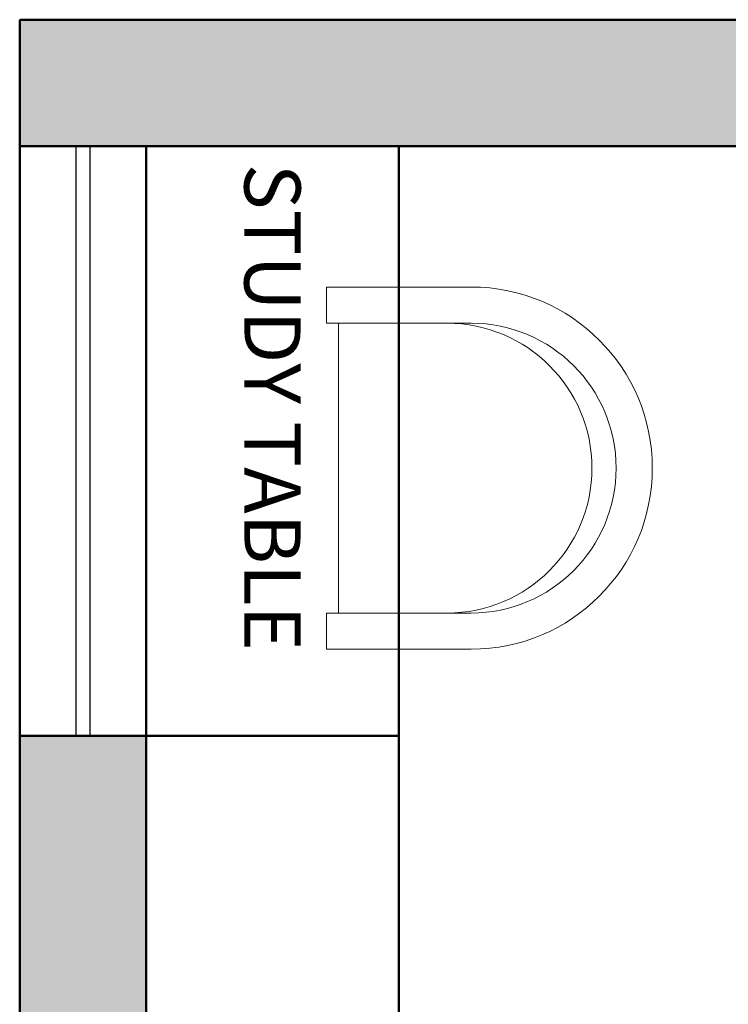
# Model space of a CAD drawing. Units: inches. Extents: x 3008 to 4088, y 1255 to 2137.
# Tile 17 of 30: x 3094 to 3144, y 1874 to 1944. Entities that reach past the tile are written whole.
import ezdxf

# ---------------------------------------------------------------- set-up
doc = ezdxf.new("R2010")
doc.units = ezdxf.units.IN
for name, color, linetype, lineweight in [('A-ANNO-TEXT', 7, 'Continuous', 18), ('A-FURN', 8, 'Continuous', 18), ('A-GLAZ', 4, 'Continuous', 25), ('A-WALL', 7, 'Continuous', 50), ('A-WALL-PATT', 8, 'Continuous', 13)]:
    doc.layers.add(name, color=color, linetype=linetype, lineweight=lineweight)
doc.styles.get("Standard").update_dxf_attribs({"font": 'arial.ttf'})

# ---------------------------------------------------------------- blocks, each defined once
blk = doc.blocks.new('12PSTG07')
at = {"color": 0, "linetype": 'ByBlock'}
for p, q in [((0, 15), (-12, 15)), ((0, 12), (0, 15)), ((-12, 12), (0, 12)), ((-1, -12), (-1, 12)), ((-12, -12), (0, -12)), ((0, -12), (0, -15)), ((0, -15), (-12, -15))]:
    blk.add_line(p, q, dxfattribs=at)
for centre, radius in [((-12, 0), 15), ((-12, 0), 12), ((-10, 0), 12)]:
    blk.add_arc(centre, radius, 90, 270, dxfattribs=at)

msp = doc.modelspace()

# ---------------------------------------------------------------- hatches: boundary and pattern name
at = {"layer": 'A-WALL-PATT'}
h = msp.add_hatch(color=256, dxfattribs=at)
h.dxf.hatch_style = 1
h.paths.add_polyline_path([(3102.666, 1625.966), (3093.666, 1625.966), (3093.666, 1540.966), (3102.666, 1540.966)])
h.paths.add_polyline_path([(3102.666, 1784.966), (3252.666, 1784.966), (3252.666, 1790.966), (3102.666, 1790.966), (3102.666, 1892.966), (3093.666, 1892.966), (3093.666, 1667.966), (3102.666, 1667.966)])
h.paths.add_polyline_path([(3192.666, 1943.966), (3093.666, 1943.966), (3093.666, 1934.966), (3102.666, 1934.966), (3192.666, 1934.966)])
h.paths.add_polyline_path([(3264.666, 1943.966), (3234.666, 1943.966), (3234.666, 1934.966), (3246.666, 1934.966), (3246.666, 1868.966), (3252.666, 1868.966), (3252.666, 1934.966), (3264.666, 1934.966)])
h.paths.add_polyline_path([(3330.666, 1943.966), (3288.666, 1943.966), (3288.666, 1934.966), (3300.666, 1934.966), (3300.666, 1838.966), (3246.666, 1838.966), (3246.666, 1826.966), (3252.666, 1826.966), (3252.666, 1832.966), (3306.666, 1832.966), (3306.666, 1934.966), (3330.666, 1934.966)])
h.paths.add_polyline_path([(3390.666, 1943.966), (3360.666, 1943.966), (3360.666, 1934.966), (3390.666, 1934.966)])
h.paths.add_polyline_path([(3465.666, 1943.966), (3432.666, 1943.966), (3432.666, 1934.966), (3456.666, 1934.966), (3456.666, 1883.966), (3465.666, 1883.966)])
h.paths.add_polyline_path([(3465.666, 1841.966), (3456.666, 1841.966), (3456.666, 1790.966), (3370.666, 1790.966), (3370.666, 1784.966), (3456.666, 1784.966), (3456.666, 1759.466), (3465.666, 1759.466)])
h.paths.add_polyline_path([(3465.666, 1693.466), (3456.666, 1693.466), (3456.666, 1667.966), (3330.666, 1667.966), (3330.666, 1643.966), (3336.666, 1643.966), (3336.666, 1661.966), (3456.666, 1661.966), (3456.666, 1649.966), (3465.666, 1649.966)])
h.paths.add_polyline_path([(3465.666, 1625.966), (3456.666, 1625.966), (3456.666, 1613.966), (3324.666, 1613.966), (3324.666, 1604.966), (3456.666, 1604.966), (3456.666, 1571.966), (3465.666, 1571.966)])
h.paths.add_polyline_path([(3465.666, 1505.966), (3456.666, 1505.966), (3456.666, 1472.966), (3438.666, 1472.966), (3438.666, 1463.966), (3465.666, 1463.966)])
h.paths.add_polyline_path([(3396.666, 1472.966), (3354.666, 1472.966), (3354.666, 1463.966), (3396.666, 1463.966)])
h.paths.add_polyline_path([(3312.666, 1472.966), (3288.666, 1472.966), (3288.666, 1550.966), (3282.666, 1550.966), (3282.666, 1472.966), (3270.666, 1472.966), (3270.666, 1463.966), (3312.666, 1463.966)])
h.paths.add_polyline_path([(3246.666, 1472.966), (3234.666, 1472.966), (3234.666, 1544.966), (3252.666, 1544.966), (3252.666, 1550.966), (3234.666, 1550.966), (3234.666, 1604.966), (3282.666, 1604.966), (3282.666, 1580.966), (3288.666, 1580.966), (3288.666, 1613.966), (3150.666, 1613.966), (3150.666, 1604.966), (3225.666, 1604.966), (3225.666, 1463.966), (3246.666, 1463.966)])

# ---------------------------------------------------------------- linework, layer by layer
at = {"layer": 'A-GLAZ'}
for p, q in [((3097.666, 1934.966), (3097.666, 1892.966)), ((3097.666, 1934.966), (3097.666, 1892.966)), ((3098.666, 1934.966), (3098.666, 1892.966))]:
    msp.add_line(p, q, dxfattribs=at)
at = {"layer": 'A-WALL'}
for p, q in [((3093.666, 1540.966), (3093.666, 1943.966)), ((3093.666, 1943.966), (3330.666, 1943.966)), ((3093.666, 1934.966), (3102.666, 1934.966)), ((3102.666, 1934.966), (3246.666, 1934.966)), ((3102.666, 1790.966), (3102.666, 1934.966)), ((3120.666, 1790.966), (3120.666, 1934.966)), ((3093.666, 1892.966), (3120.666, 1892.966))]:
    msp.add_line(p, q, dxfattribs=at)

# ---------------------------------------------------------------- block references
at = {"layer": 'A-FURN', "xscale": 0.8597921787217941, "yscale": 0.8597921787217941, "zscale": 0.8597921787217941, "rotation": 180}
msp.add_blockref('12PSTG07', (3115.507, 1912.032), dxfattribs=at)

# ---------------------------------------------------------------- texts
at = {"layer": 'A-ANNO-TEXT', "insert": (3113.669, 1933.701), "char_height": 4, "attachment_point": 1, "rotation": 270}
msp.add_mtext_dynamic_manual_height_columns('{\\fTimes New Roman|b0|i0|c0|p18;STUDY TABLE}', width=105.61268, gutter_width=12.5, heights=[0], dxfattribs=at)

doc.saveas('drawing.dxf')
